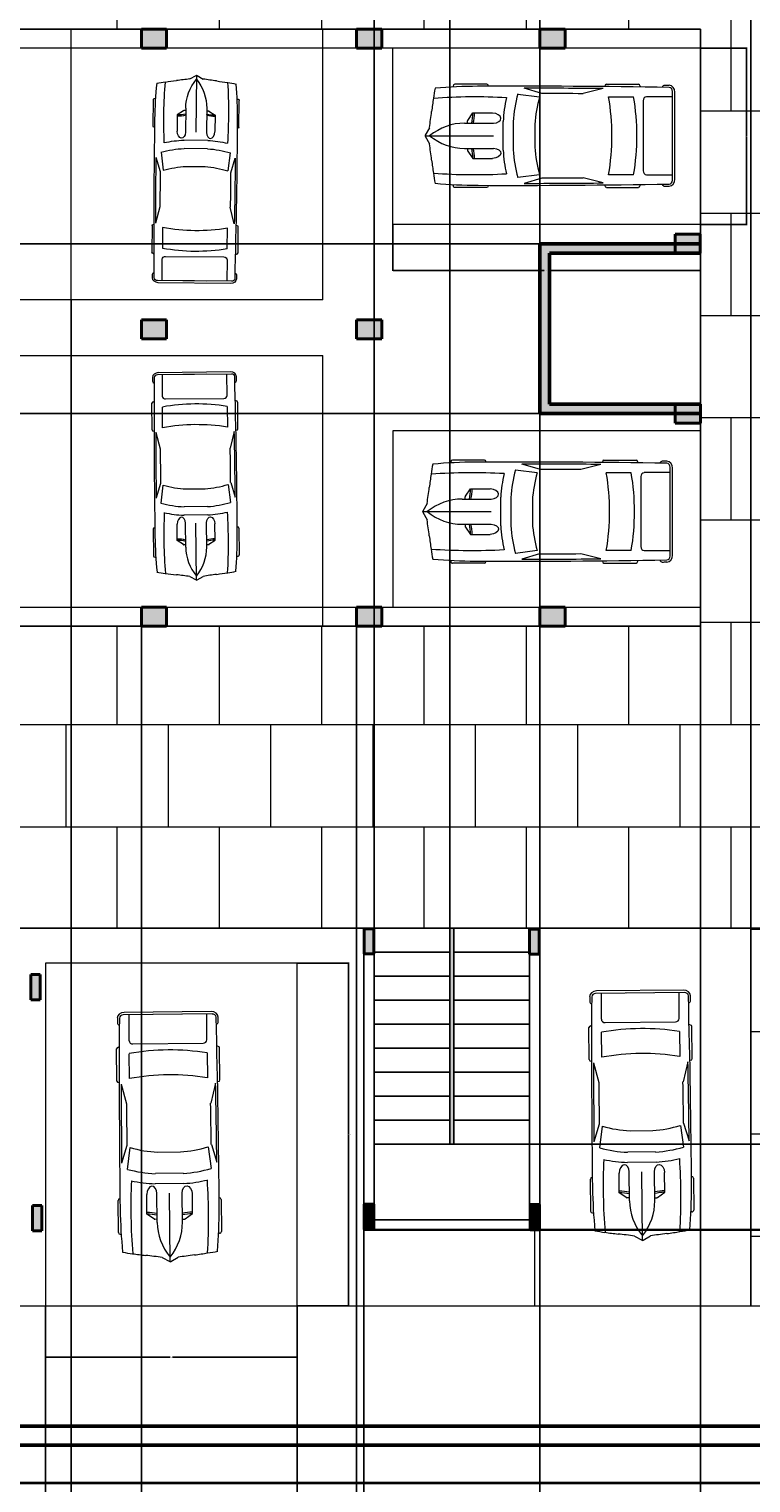
# Model space of a CAD drawing. Units: inches. Extents: x 154617 to 156384, y 250671 to 252576.
# Tile 4 of 6: x 155601 to 155945, y 251035 to 251728. Entities that reach past the tile are written whole.
import ezdxf

# ---------------------------------------------------------------- set-up
doc = ezdxf.new("R2010")
doc.units = ezdxf.units.IN
for name, color, linetype, lineweight in [('A-ANNO-DIMS', 2, 'Continuous', 18), ('A-COLS-PATT', 6, 'Continuous', 13), ('A-EQPM-VEHI', 9, 'Continuous', 13), ('A-FLOR-DRIV', 5, 'Continuous', 25), ('A-FLOR-PATT', 112, 'Continuous', 13), ('A-FLOR-PRKG', 4, 'Continuous', 18), ('A-FLOR-STRS', 7, 'Continuous', 25), ('A-FLOR-STRS-PATT', 20, 'Continuous', 13), ('A-WALL-PATT', 8, 'Continuous', 13), ('C-PROP', 5, 'Continuous', 35), ('pillars', 6, 'Continuous', 40), ('walls', 4, 'Continuous', 50)]:
    doc.layers.add(name, color=color, linetype=linetype, lineweight=lineweight)
doc.styles.get("Standard").update_dxf_attribs({"font": 'arial.ttf'})
doc.dimstyles.get("Standard").update_dxf_attribs({"dimtxt": 0.18, "dimasz": 0.18, "dimexe": 0.18, "dimexo": 0.0625, "dimgap": 0.09, "dimtad": 0, "dimtih": 1, "dimtoh": 1, "dimdec": 4, "dimzin": 0, "dimdsep": 46, "dimtxsty": 'Standard', "dimcen": 0.09, "dimadec": 0, "dimazin": 0, "dimtfac": 1, "dimtdec": 4, "dimtofl": 0, "dimtmove": 0, "dimatfit": 3, "dimfxl": 1, "dimtolj": 1, "dimtzin": 0, "dimarcsym": 0})

# ---------------------------------------------------------------- blocks, each defined once
blk = doc.blocks.new('*U2')
for p, q in [((21.1, 37.4), (21.1, 36.8)), ((46.6, 38.9), (22.4, 38.9)), ((47.8, 37.4), (47.8, 37.4)), ((88, 31.9), (74.8, 35.9)), ((134.3, 35.6), (119.3, 31.8)), ((135.5, 37.1), (135.5, 37.4)), ((136.7, 38.9), (160.9, 38.9)), ((162.1, 37.4), (162.1, 36.8)), ((186.5, -33.5), (186.5, 33.5)), ((70, 31.5), (86.4, 29.4)), ((138.4, 29.4), (157.2, 29.4)), ((164.5, 26.4), (164.5, -26.4)), ((186.5, 29.4), (167, 29.4)), ((188.4, -32.8), (188.4, 32.8)), ((32.1, 9.5), (32.1, 11.2)), ((32.3, 11.6), (36.1, 17.2)), ((36.1, 17.2), (50.9, 17.2)), ((3.3, 6.1), (0.1, 0.4)), ((29.8, 9.5), (51.7, 9.5)), ((58.9, -10.8), (58.9, 10.8)), ((66.6, -10.5), (66.6, 10.5)), ((82.7, 8.5), (82.7, -8.5)), ((186.5, -10.5), (186.5, 10.5)), ((0, 0), (51.7, 0)), ((0.1, -0.4), (3.3, -6.1)), ((29.8, -9.5), (51.7, -9.5)), ((32.1, -9.5), (32.1, -11.2)), ((32.3, -11.6), (36.1, -17.2)), ((36.1, -17.2), (50.9, -17.2)), ((86.4, -29.4), (70, -31.5)), ((88, -31.9), (74.8, -35.9)), ((134.3, -35.6), (119.3, -31.8)), ((157.2, -29.4), (138.4, -29.4)), ((167, -29.4), (186.5, -29.4)), ((21.1, -37.4), (21.1, -36.8)), ((46.6, -38.9), (22.4, -38.9)), ((47.8, -37.4), (47.8, -37.4)), ((135.5, -37.1), (135.5, -37.4)), ((136.7, -38.9), (160.9, -38.9)), ((162.1, -37.4), (162.1, -36.8))]:
    blk.add_line(p, q)
for centre, major_axis, ratio, start_param, end_param in [((266, -27.5), (0, 313.3), 0.842304, 1.367076, 1.39176), ((41.2, -490.9), (0, 528.2), 0.842304, 0.00281, 0.075598), ((22.4, 37.4), (0, -1.48), 0.842304, 3.141593, 4.712389), ((64.5, -10555.6), (0, 10593), 0.842304, -0.013397, 0.002797), ((46.6, 37.4), (0, 1.48), 0.842304, -1.570796, 0), ((64.5, -10555.6), (0, -10591.5), 0.842304, 3.133765, 3.140441), ((136.7, 37.4), (0, -1.48), 0.842304, 3.141593, 4.712389), ((160.9, 37.4), (0, 1.48), 0.842304, -1.570796, 0), ((180.6, 35.8), (0, 2.22), 0.842304, -0.013017, 1.249894), ((64.5, -10556.4), (0, 10595.3), 0.842304, -0.013397, -0.013017), ((184, 32.8), (0, -5.25), 0.842304, 1.570796, 3.128196), ((184, 33.5), (0, -2.96), 0.842304, 1.570796, 3.128196), ((259.2, -27.5), (0, -305.3), 0.842304, 4.528606, 4.561838), ((37.5, -594), (0, -623.3), 0.842304, 3.096046, 3.200911), ((134.4, 5.4), (0, -89.8), 0.842304, 4.449482, 4.652344), ((135.3, 5.4), (0, 81.8), 0.842304, 1.245306, 1.50788), ((149.6, 2.8), (0, -79.6), 0.842304, 4.372215, 4.640744), ((95.8, -3666.4), (0, -3698.2), 0.842304, 3.134049, 3.144098), ((17.1, 0), (0, 147), 0.842304, 4.511394, 4.913384), ((35.9, 0), (0, 147), 0.842304, 4.511394, 4.913384), ((167, 26.4), (0, 2.96), 0.842304, 0, 1.570796), ((-204.5, 52.4), (0, -251), 0.842304, 1.385369, 1.434372), ((32.7, 11.2), (0, 0.74), 0.842304, 0.879714, 1.570796), ((13, 17), (0, 27.4), 0.842304, 4.435146, 4.718221), ((14.2, 17), (0, 27.4), 0.842304, 4.435146, 4.718221), ((50.8, 13.3), (6.34, -0.36), 0.603834, -1.395552, 1.581315), ((0.6, 0), (0, -0.74), 0.842304, 4.131459, 5.293319), ((29.8, -46.7), (0, 56.2), 0.842304, 0, 0.590319), ((-204.5, -52.4), (0, 251), 0.842304, -1.434372, -1.385369), ((29.8, 46.7), (0, 56.2), 0.842304, 2.551274, 3.141593), ((13, -17), (0, -27.4), 0.842304, 1.564964, 1.848039), ((14.2, -17), (0, -27.4), 0.842304, 1.564964, 1.848039), ((134.4, -5.4), (0, -89.8), 0.842304, -1.510751, -1.307889), ((135.3, -5.4), (0, -81.8), 0.842304, -1.50788, -1.245306), ((149.6, -2.8), (0, -79.6), 0.842304, -1.499151, -1.230623), ((259.2, 27.5), (0, 305.3), 0.842304, 1.721348, 1.754579), ((32.7, -11.2), (0, -0.74), 0.842304, 4.712389, 5.403472), ((266, 27.5), (0, 313.3), 0.842304, 1.749832, 1.774517), ((37.5, 594), (0, -623.3), 0.842304, -0.059319, 0.045547), ((95.8, 3666.4), (0, -3698.2), 0.842304, -0.002505, 0.007544), ((167, -26.4), (0, -2.96), 0.842304, 4.712389, 6.283185), ((184, -32.8), (0, -5.25), 0.842304, 0.013397, 1.570796), ((41.2, 490.9), (0, -528.2), 0.842304, -0.075598, -0.00281), ((22.4, -37.4), (0, 1.48), 0.842304, 1.570796, 3.141593), ((64.5, 10555.6), (0, 10593), 0.842304, 3.138796, 3.15499), ((46.6, -37.4), (0, -1.48), 0.842304, 0, 1.570796), ((64.5, 10555.6), (0, -10591.5), 0.842304, 0.001152, 0.007828), ((136.7, -37.4), (0, -1.48), 0.842304, -1.570796, 0), ((160.9, -37.4), (0, 1.48), 0.842304, 3.141593, 4.712389), ((180.6, -35.8), (0, -2.22), 0.842304, -1.249894, 0.013017), ((64.5, 10556.4), (0, 10595.3), 0.842304, 3.15461, 3.15499), ((184, -33.5), (0, 2.96), 0.842304, 3.15499, 4.712389)]:
    blk.add_ellipse(centre, major_axis=major_axis, ratio=ratio, start_param=start_param, end_param=end_param)
at = {"extrusion": (0, 0, -1)}
blk.add_ellipse((50.8, -13.3), major_axis=(6.34, 0.36), ratio=0.603834, start_param=-1.395552, end_param=1.581315, dxfattribs=at)
blk = doc.blocks.new('COL-RECT-12x9')
h = blk.add_hatch(color=256)
h.dxf.hatch_style = 1
h.paths.add_polyline_path([(12.01, 0), (12.01, 9), (0, 9), (0, 0)])
for p, q in [((12.01, 9), (0, 9)), ((0, 9), (0, 0)), ((12.01, 0), (12.01, 9)), ((0, 0), (12.01, 0))]:
    blk.add_line(p, q)
blk = doc.blocks.new('COL-NARROW-4_5x12')
h = blk.add_hatch(color=256)
h.dxf.hatch_style = 1
h.paths.add_polyline_path([(4.5, 12.01), (0, 12.01), (0, 0), (4.5, 0)])
for p, q in [((4.5, 12.01), (0, 12.01)), ((0, 12.01), (0, 0)), ((4.5, 0), (4.5, 12.01)), ((0, 0), (4.5, 0))]:
    blk.add_line(p, q)
blk = doc.blocks.new('PARKING-BAY-U')
for p, q in [((120, 163.22), (0, 163.22)), ((0, 163.22), (0, 0)), ((120, 0), (120, 163.22))]:
    blk.add_line(p, q)
blk = doc.blocks.new('PARKING-BAY-L')
for p, q in [((0, 0), (0, 84)), ((146.69, 0), (0, 0))]:
    blk.add_line(p, q)
blk = doc.blocks.new('*D15')
at = {"layer": 'A-ANNO-DIMS', "color": 0, "lineweight": -2, "transparency": 16777216}
for p, q in [((155728.99, 251282.75), (155753.59, 251282.75)), ((155753.41, 251282.57), (155753.41, 251201.32)), ((155753.41, 251119.71), (155753.41, 251200.96)), ((155728.99, 251119.53), (155753.59, 251119.53))]:
    blk.add_line(p, q, dxfattribs=at)
at = {"layer": 'A-ANNO-DIMS', "color": 0, "transparency": 16777216}
for points in [[(155753.38, 251282.57), (155753.44, 251282.57), (155753.41, 251282.75)], [(155753.38, 251119.71), (155753.44, 251119.71), (155753.41, 251119.53)]]:
    blk.add_solid(points, dxfattribs=at)
at = {"layer": 'Defpoints', "color": 0, "transparency": 16777216}
for p in [(155728.93, 251282.75), (155753.41, 251282.75), (155728.93, 251119.53)]:
    blk.add_point(p, dxfattribs=at)
at = {"layer": 'A-ANNO-DIMS', "color": 0, "transparency": 16777216, "insert": (155753.41, 251201.14), "char_height": 0.18, "attachment_point": 5}
blk.add_mtext('\\A1;END BAY 163 TYP.', dxfattribs=at)
blk = doc.blocks.new('*D16')
at = {"layer": 'A-ANNO-DIMS', "color": 0, "lineweight": -2, "transparency": 16777216}
for p, q in [((155608.93, 251119.46), (155608.93, 251094.86)), ((155728.93, 251119.46), (155728.93, 251094.86)), ((155609.11, 251095.04), (155668.34, 251095.04)), ((155728.75, 251095.04), (155669.52, 251095.04))]:
    blk.add_line(p, q, dxfattribs=at)
at = {"layer": 'A-ANNO-DIMS', "color": 0, "transparency": 16777216}
for points in [[(155609.11, 251095.07), (155609.11, 251095.01), (155608.93, 251095.04)], [(155728.75, 251095.07), (155728.75, 251095.01), (155728.93, 251095.04)]]:
    blk.add_solid(points, dxfattribs=at)
at = {"layer": 'Defpoints', "color": 0, "transparency": 16777216}
for p in [(155608.93, 251119.53), (155728.93, 251119.53), (155728.93, 251095.04)]:
    blk.add_point(p, dxfattribs=at)
at = {"layer": 'A-ANNO-DIMS', "color": 0, "transparency": 16777216, "insert": (155668.93, 251095.04), "char_height": 0.18, "attachment_point": 5}
blk.add_mtext('\\A1;120 TYP.', dxfattribs=at)
blk = doc.blocks.new('*D17')
at = {"layer": 'A-ANNO-DIMS', "color": 0, "lineweight": -2, "transparency": 16777216}
for p, q in [((155774.41, 251634.96), (155774.41, 251612.84)), ((155921.1, 251634.96), (155921.1, 251612.84)), ((155774.59, 251613.02), (155846.54, 251613.02)), ((155920.92, 251613.02), (155848.96, 251613.02))]:
    blk.add_line(p, q, dxfattribs=at)
at = {"layer": 'A-ANNO-DIMS', "color": 0, "transparency": 16777216}
for points in [[(155774.59, 251613.05), (155774.59, 251612.99), (155774.41, 251613.02)], [(155920.92, 251613.05), (155920.92, 251612.99), (155921.1, 251613.02)]]:
    blk.add_solid(points, dxfattribs=at)
at = {"layer": 'Defpoints', "color": 0, "transparency": 16777216}
for p in [(155774.41, 251635.03), (155921.1, 251635.03), (155921.1, 251613.02)]:
    blk.add_point(p, dxfattribs=at)
at = {"layer": 'A-ANNO-DIMS', "color": 0, "transparency": 16777216, "insert": (155847.75, 251613.02), "char_height": 0.18, "attachment_point": 5}
blk.add_mtext('\\A1;SIDE BAY 147 TYP.', dxfattribs=at)
blk = doc.blocks.new('*D18')
at = {"layer": 'A-ANNO-DIMS', "color": 0, "lineweight": -2, "transparency": 16777216}
for p, q in [((155921.16, 251719.03), (155943.28, 251719.03)), ((155943.1, 251718.85), (155943.1, 251677.21)), ((155943.1, 251635.21), (155943.1, 251676.84)), ((155921.16, 251635.03), (155943.28, 251635.03))]:
    blk.add_line(p, q, dxfattribs=at)
at = {"layer": 'A-ANNO-DIMS', "color": 0, "transparency": 16777216}
for points in [[(155943.07, 251718.85), (155943.13, 251718.85), (155943.1, 251719.03)], [(155943.07, 251635.21), (155943.13, 251635.21), (155943.1, 251635.03)]]:
    blk.add_solid(points, dxfattribs=at)
at = {"layer": 'Defpoints', "color": 0, "transparency": 16777216}
for p in [(155921.1, 251719.03), (155943.1, 251719.03), (155921.1, 251635.03)]:
    blk.add_point(p, dxfattribs=at)
at = {"layer": 'A-ANNO-DIMS', "color": 0, "transparency": 16777216, "insert": (155943.1, 251677.03), "char_height": 0.18, "attachment_point": 5}
blk.add_mtext('\\A1;84 TYP.', dxfattribs=at)
blk = doc.blocks.new('*D37')
at = {"layer": 'A-ANNO-DIMS', "color": 0, "lineweight": -2, "transparency": 16777216}
for p, q in [((155475.98, 251443.46), (155475.98, 250671.2)), ((155654.61, 251443.46), (155654.61, 250671.2)), ((155476.16, 250671.38), (155564.84, 250671.38)), ((155654.43, 250671.38), (155565.75, 250671.38))]:
    blk.add_line(p, q, dxfattribs=at)
at = {"layer": 'A-ANNO-DIMS', "color": 0, "transparency": 16777216}
for points in [[(155476.16, 250671.41), (155476.16, 250671.35), (155475.98, 250671.38)], [(155654.43, 250671.41), (155654.43, 250671.35), (155654.61, 250671.38)]]:
    blk.add_solid(points, dxfattribs=at)
at = {"layer": 'Defpoints', "color": 0, "transparency": 16777216}
for p in [(155475.98, 251443.53), (155654.61, 251443.53), (155654.61, 250671.38)]:
    blk.add_point(p, dxfattribs=at)
at = {"layer": 'A-ANNO-DIMS', "color": 0, "transparency": 16777216, "insert": (155565.3, 250671.38), "char_height": 0.18, "attachment_point": 5}
blk.add_mtext('\\A1;178.63', dxfattribs=at)
blk = doc.blocks.new('*D38')
at = {"layer": 'A-ANNO-DIMS', "color": 0, "lineweight": -2, "transparency": 16777216}
for p, q in [((155654.61, 251443.46), (155654.61, 250671.2)), ((155757.2, 251443.46), (155757.2, 250671.2)), ((155654.79, 250671.38), (155705.45, 250671.38)), ((155757.02, 250671.38), (155706.36, 250671.38))]:
    blk.add_line(p, q, dxfattribs=at)
at = {"layer": 'A-ANNO-DIMS', "color": 0, "transparency": 16777216}
for points in [[(155654.79, 250671.41), (155654.79, 250671.35), (155654.61, 250671.38)], [(155757.02, 250671.41), (155757.02, 250671.35), (155757.2, 250671.38)]]:
    blk.add_solid(points, dxfattribs=at)
at = {"layer": 'Defpoints', "color": 0, "transparency": 16777216}
for p in [(155654.61, 251443.53), (155757.2, 251443.53), (155757.2, 250671.38)]:
    blk.add_point(p, dxfattribs=at)
at = {"layer": 'A-ANNO-DIMS', "color": 0, "transparency": 16777216, "insert": (155705.91, 250671.38), "char_height": 0.18, "attachment_point": 5}
blk.add_mtext('\\A1;102.59', dxfattribs=at)
blk = doc.blocks.new('*D39')
at = {"layer": 'A-ANNO-DIMS', "color": 0, "lineweight": -2, "transparency": 16777216}
for p, q in [((155757.2, 251443.46), (155757.2, 250671.2)), ((155844.6, 251443.46), (155844.6, 250671.2)), ((155757.38, 250671.38), (155800.58, 250671.38)), ((155844.42, 250671.38), (155801.22, 250671.38))]:
    blk.add_line(p, q, dxfattribs=at)
at = {"layer": 'A-ANNO-DIMS', "color": 0, "transparency": 16777216}
for points in [[(155757.38, 250671.41), (155757.38, 250671.35), (155757.2, 250671.38)], [(155844.42, 250671.41), (155844.42, 250671.35), (155844.6, 250671.38)]]:
    blk.add_solid(points, dxfattribs=at)
at = {"layer": 'Defpoints', "color": 0, "transparency": 16777216}
for p in [(155757.2, 251443.53), (155844.6, 251443.53), (155844.6, 250671.38)]:
    blk.add_point(p, dxfattribs=at)
at = {"layer": 'A-ANNO-DIMS', "color": 0, "transparency": 16777216, "insert": (155800.9, 250671.38), "char_height": 0.18, "attachment_point": 5}
blk.add_mtext('\\A1;87.4', dxfattribs=at)
blk = doc.blocks.new('*D52')
at = {"layer": 'A-ANNO-DIMS', "color": 0, "lineweight": -2, "transparency": 16777216}
for p, q in [((155760.6, 251155.46), (155760.6, 250671.2)), ((155844.6, 251155.46), (155844.6, 250671.2)), ((155760.78, 250671.38), (155802.38, 250671.38)), ((155844.42, 250671.38), (155802.82, 250671.38))]:
    blk.add_line(p, q, dxfattribs=at)
at = {"layer": 'A-ANNO-DIMS', "color": 0, "transparency": 16777216}
for points in [[(155760.78, 250671.41), (155760.78, 250671.35), (155760.6, 250671.38)], [(155844.42, 250671.41), (155844.42, 250671.35), (155844.6, 250671.38)]]:
    blk.add_solid(points, dxfattribs=at)
at = {"layer": 'Defpoints', "color": 0, "transparency": 16777216}
for p in [(155760.6, 251155.53), (155844.6, 251155.53), (155844.6, 250671.38)]:
    blk.add_point(p, dxfattribs=at)
at = {"layer": 'A-ANNO-DIMS', "color": 0, "transparency": 16777216, "insert": (155802.6, 250671.38), "char_height": 0.18, "attachment_point": 5}
blk.add_mtext('\\A1;84', dxfattribs=at)
blk = doc.blocks.new('*D53')
at = {"layer": 'A-ANNO-DIMS', "color": 0, "lineweight": -2, "transparency": 16777216}
for p, q in [((155844.66, 251299.53), (156383.38, 251299.53)), ((156383.2, 251299.35), (156383.2, 251227.71)), ((156383.2, 251155.71), (156383.2, 251227.35)), ((155844.66, 251155.53), (156383.38, 251155.53))]:
    blk.add_line(p, q, dxfattribs=at)
at = {"layer": 'A-ANNO-DIMS', "color": 0, "transparency": 16777216}
for points in [[(156383.17, 251299.35), (156383.23, 251299.35), (156383.2, 251299.53)], [(156383.17, 251155.71), (156383.23, 251155.71), (156383.2, 251155.53)]]:
    blk.add_solid(points, dxfattribs=at)
at = {"layer": 'Defpoints', "color": 0, "transparency": 16777216}
for p in [(155844.6, 251299.53), (156383.2, 251299.53), (155844.6, 251155.53)]:
    blk.add_point(p, dxfattribs=at)
at = {"layer": 'A-ANNO-DIMS', "color": 0, "transparency": 16777216, "insert": (156383.2, 251227.53), "char_height": 0.18, "attachment_point": 5}
blk.add_mtext('\\A1;144', dxfattribs=at)
blk = doc.blocks.new('*D54')
at = {"layer": 'A-ANNO-DIMS', "color": 0, "lineweight": -2, "transparency": 16777216}
for p, q in [((155844.6, 251544.74), (155844.6, 250671.2)), ((155921.1, 251544.74), (155921.1, 250671.2)), ((155844.78, 250671.38), (155882.52, 250671.38)), ((155920.92, 250671.38), (155883.17, 250671.38))]:
    blk.add_line(p, q, dxfattribs=at)
at = {"layer": 'A-ANNO-DIMS', "color": 0, "transparency": 16777216}
for points in [[(155844.78, 250671.41), (155844.78, 250671.35), (155844.6, 250671.38)], [(155920.92, 250671.41), (155920.92, 250671.35), (155921.1, 250671.38)]]:
    blk.add_solid(points, dxfattribs=at)
at = {"layer": 'Defpoints', "color": 0, "transparency": 16777216}
for p in [(155844.6, 251544.8), (155921.1, 251544.8), (155921.1, 250671.38)]:
    blk.add_point(p, dxfattribs=at)
at = {"layer": 'A-ANNO-DIMS', "color": 0, "transparency": 16777216, "insert": (155882.85, 250671.38), "char_height": 0.18, "attachment_point": 5}
blk.add_mtext('\\A1;76.5', dxfattribs=at)
blk = doc.blocks.new('*D55')
at = {"layer": 'A-ANNO-DIMS', "color": 0, "lineweight": -2, "transparency": 16777216}
for p, q in [((155844.53, 251625.8), (154616.73, 251625.8)), ((154616.91, 251625.62), (154616.91, 251585.48)), ((154616.91, 251544.98), (154616.91, 251585.12)), ((155844.53, 251544.8), (154616.73, 251544.8))]:
    blk.add_line(p, q, dxfattribs=at)
at = {"layer": 'A-ANNO-DIMS', "color": 0, "transparency": 16777216}
for points in [[(154616.88, 251625.62), (154616.94, 251625.62), (154616.91, 251625.8)], [(154616.88, 251544.98), (154616.94, 251544.98), (154616.91, 251544.8)]]:
    blk.add_solid(points, dxfattribs=at)
at = {"layer": 'Defpoints', "color": 0, "transparency": 16777216}
for p in [(154616.91, 251625.8), (155844.6, 251625.8), (155844.6, 251544.8)]:
    blk.add_point(p, dxfattribs=at)
at = {"layer": 'A-ANNO-DIMS', "color": 0, "transparency": 16777216, "insert": (154616.91, 251585.3), "char_height": 0.18, "attachment_point": 5}
blk.add_mtext('\\A1;81', dxfattribs=at)
blk = doc.blocks.new('*D57')
at = {"layer": 'A-ANNO-DIMS', "color": 0, "lineweight": -2, "transparency": 16777216}
for p, q in [((155480.24, 251119.46), (155480.24, 250671.2)), ((155608.93, 251119.46), (155608.93, 250671.2)), ((155480.42, 250671.38), (155544.13, 250671.38)), ((155608.75, 250671.38), (155545.04, 250671.38))]:
    blk.add_line(p, q, dxfattribs=at)
at = {"layer": 'A-ANNO-DIMS', "color": 0, "transparency": 16777216}
for points in [[(155480.42, 250671.41), (155480.42, 250671.35), (155480.24, 250671.38)], [(155608.75, 250671.41), (155608.75, 250671.35), (155608.93, 250671.38)]]:
    blk.add_solid(points, dxfattribs=at)
at = {"layer": 'Defpoints', "color": 0, "transparency": 16777216}
for p in [(155480.24, 251119.53), (155608.93, 251119.53), (155608.93, 250671.38)]:
    blk.add_point(p, dxfattribs=at)
at = {"layer": 'A-ANNO-DIMS', "color": 0, "transparency": 16777216, "insert": (155544.58, 250671.38), "char_height": 0.18, "attachment_point": 5}
blk.add_mtext('\\A1;128.68', dxfattribs=at)
blk = doc.blocks.new('*D58')
at = {"layer": 'A-ANNO-DIMS', "color": 0, "lineweight": -2, "transparency": 16777216}
for p, q in [((155844.6, 251299.59), (155844.6, 252576.18)), ((155844.78, 252576), (155894.46, 252576)), ((155944.92, 252576), (155895.23, 252576)), ((155945.1, 251299.59), (155945.1, 252576.18))]:
    blk.add_line(p, q, dxfattribs=at)
at = {"layer": 'A-ANNO-DIMS', "color": 0, "transparency": 16777216}
for points in [[(155844.78, 252576.03), (155844.78, 252575.97), (155844.6, 252576)], [(155944.92, 252576.03), (155944.92, 252575.97), (155945.1, 252576)]]:
    blk.add_solid(points, dxfattribs=at)
at = {"layer": 'Defpoints', "color": 0, "transparency": 16777216}
for p in [(155945.1, 252576), (155844.6, 251299.53), (155945.1, 251299.53)]:
    blk.add_point(p, dxfattribs=at)
at = {"layer": 'A-ANNO-DIMS', "color": 0, "transparency": 16777216, "insert": (155894.85, 252576), "char_height": 0.18, "attachment_point": 5}
blk.add_mtext('\\A1;100.5', dxfattribs=at)
blk = doc.blocks.new('*D61')
at = {"layer": 'A-ANNO-DIMS', "color": 0, "lineweight": -2, "transparency": 16777216}
for p, q in [((155501.1, 251598.96), (155501.1, 250671.2)), ((155621.1, 251598.96), (155621.1, 250671.2)), ((155501.28, 250671.38), (155560.82, 250671.38)), ((155620.92, 250671.38), (155561.38, 250671.38))]:
    blk.add_line(p, q, dxfattribs=at)
at = {"layer": 'A-ANNO-DIMS', "color": 0, "transparency": 16777216}
for points in [[(155501.28, 250671.41), (155501.28, 250671.35), (155501.1, 250671.38)], [(155620.92, 250671.41), (155620.92, 250671.35), (155621.1, 250671.38)]]:
    blk.add_solid(points, dxfattribs=at)
at = {"layer": 'Defpoints', "color": 0, "transparency": 16777216}
for p in [(155501.1, 251599.03), (155621.1, 251599.03), (155621.1, 250671.38)]:
    blk.add_point(p, dxfattribs=at)
at = {"layer": 'A-ANNO-DIMS', "color": 0, "transparency": 16777216, "insert": (155561.1, 250671.38), "char_height": 0.18, "attachment_point": 5}
blk.add_mtext('\\A1;120', dxfattribs=at)
blk = doc.blocks.new('*D68')
at = {"layer": 'A-ANNO-DIMS', "color": 0, "lineweight": -2, "transparency": 16777216}
for p, q in [((155760.6, 251155.46), (155760.6, 250671.2)), ((155728.93, 251119.46), (155728.93, 250671.2)), ((155729.11, 250671.38), (155744.37, 250671.38)), ((155760.42, 250671.38), (155745.16, 250671.38))]:
    blk.add_line(p, q, dxfattribs=at)
at = {"layer": 'A-ANNO-DIMS', "color": 0, "transparency": 16777216}
for points in [[(155729.11, 250671.41), (155729.11, 250671.35), (155728.93, 250671.38)], [(155760.42, 250671.41), (155760.42, 250671.35), (155760.6, 250671.38)]]:
    blk.add_solid(points, dxfattribs=at)
at = {"layer": 'Defpoints', "color": 0, "transparency": 16777216}
for p in [(155760.6, 251155.53), (155728.93, 251119.53), (155760.6, 250671.38)]:
    blk.add_point(p, dxfattribs=at)
at = {"layer": 'A-ANNO-DIMS', "color": 0, "transparency": 16777216, "insert": (155744.76, 250671.38), "char_height": 0.18, "attachment_point": 5}
blk.add_mtext('\\A1;31.67', dxfattribs=at)
blk = doc.blocks.new('*D69')
at = {"layer": 'A-ANNO-DIMS', "color": 0, "lineweight": -2, "transparency": 16777216}
for p, q in [((155765.66, 251196.53), (156383.38, 251196.53)), ((156383.2, 251196.35), (156383.2, 251176.37)), ((156383.2, 251156.03), (156383.2, 251176.01)), ((155765.41, 251155.85), (156383.38, 251155.85))]:
    blk.add_line(p, q, dxfattribs=at)
at = {"layer": 'A-ANNO-DIMS', "color": 0, "transparency": 16777216}
for points in [[(156383.17, 251196.35), (156383.23, 251196.35), (156383.2, 251196.53)], [(156383.17, 251156.03), (156383.23, 251156.03), (156383.2, 251155.85)]]:
    blk.add_solid(points, dxfattribs=at)
at = {"layer": 'Defpoints', "color": 0, "transparency": 16777216}
for p in [(155765.6, 251196.53), (156383.2, 251196.53), (155765.34, 251155.85)]:
    blk.add_point(p, dxfattribs=at)
at = {"layer": 'A-ANNO-DIMS', "color": 0, "transparency": 16777216, "insert": (156383.2, 251176.19), "char_height": 0.18, "attachment_point": 5}
blk.add_mtext('\\A1;40.67', dxfattribs=at)
blk = doc.blocks.new('*D70')
at = {"layer": 'A-ANNO-DIMS', "color": 0, "lineweight": -2, "transparency": 16777216}
for p, q in [((155765.6, 251299.59), (155765.6, 252576.18)), ((155765.78, 252576), (155783.38, 252576)), ((155801.42, 252576), (155783.82, 252576)), ((155801.6, 251299.59), (155801.6, 252576.18))]:
    blk.add_line(p, q, dxfattribs=at)
at = {"layer": 'A-ANNO-DIMS', "color": 0, "transparency": 16777216}
for points in [[(155765.78, 252576.03), (155765.78, 252575.97), (155765.6, 252576)], [(155801.42, 252576.03), (155801.42, 252575.97), (155801.6, 252576)]]:
    blk.add_solid(points, dxfattribs=at)
at = {"layer": 'Defpoints', "color": 0, "transparency": 16777216}
for p in [(155801.6, 252576), (155765.6, 251299.53), (155801.6, 251299.53)]:
    blk.add_point(p, dxfattribs=at)
at = {"layer": 'A-ANNO-DIMS', "color": 0, "transparency": 16777216, "insert": (155783.6, 252576), "char_height": 0.18, "attachment_point": 5}
blk.add_mtext('\\A1;36', dxfattribs=at)

msp = doc.modelspace()

# ---------------------------------------------------------------- hatches: boundary and pattern name
at = {"layer": 'A-COLS-PATT'}
h = msp.add_hatch(color=256, dxfattribs=at)
h.dxf.hatch_style = 1
h.paths.add_polyline_path([(155921.015, 251630.322), (155909.002, 251630.322), (155909.002, 251625.802), (155921.015, 251625.802)])
h = msp.add_hatch(color=256, dxfattribs=at)
h.dxf.hatch_style = 1
h.paths.add_polyline_path([(155921.07, 251544.802), (155909.057, 251544.802), (155909.057, 251540.302), (155921.07, 251540.302)])
h = msp.add_hatch(color=256, dxfattribs=at)
h.dxf.hatch_style = 1
h.paths.add_polyline_path([(155765.343, 251167.865), (155760.843, 251167.865), (155760.843, 251160.526), (155765.343, 251160.526)])
h = msp.add_hatch(color=256, dxfattribs=at)
h.dxf.hatch_style = 1
h.paths.add_polyline_path([(155844.407, 251167.728), (155839.907, 251167.728), (155839.907, 251160.526), (155844.407, 251160.526)])
h = msp.add_hatch(color=256, dxfattribs=at)
h.dxf.hatch_style = 1
h.paths.add_polyline_path([(155765.343, 251160.526), (155760.843, 251160.526), (155760.843, 251155.853), (155765.343, 251155.853)])
h = msp.add_hatch(color=256, dxfattribs=at)
h.dxf.hatch_style = 1
h.paths.add_polyline_path([(155844.407, 251160.526), (155839.907, 251160.526), (155839.907, 251155.715), (155844.407, 251155.715)])
at = {"layer": 'A-FLOR-PATT'}
h = msp.add_hatch(dxfattribs=at)
h.set_pattern_fill('AR-B88', color=256, scale=0.24)
h.set_pattern_definition([(0, (0, -2.5), (0, 48.768), []), (90, (0, -2.5), (-24.384, 48.768), [48.768, -48.768])])
h.paths.add_polyline_path([(155324.842, 251443.526), (155324.842, 251299.526), (155945.097, 251299.526), (155945.097, 251119.526), (156089.097, 251119.526), (156089.097, 252132.026), (155921.097, 252132.026), (155921.097, 251872.026), (155324.842, 251872.026), (155324.842, 251728.026), (155921.097, 251728.026), (155921.097, 251443.526)])
at = {"layer": 'A-FLOR-STRS-PATT'}
h = msp.add_hatch(color=256, dxfattribs=at)
h.dxf.hatch_style = 1
h.paths.add_polyline_path([(155803.597, 251299.526), (155801.597, 251299.526), (155801.597, 251196.526), (155803.597, 251196.526)])
at = {"layer": 'A-WALL-PATT'}
h = msp.add_hatch(color=256, dxfattribs=at)
h.dxf.hatch_style = 1
h.paths.add_polyline_path([(155921.097, 251549.302), (155849.097, 251549.302), (155849.097, 251621.302), (155921.097, 251621.302), (155921.097, 251625.802), (155844.597, 251625.802), (155844.597, 251544.802), (155921.097, 251544.802)])

# ---------------------------------------------------------------- linework, layer by layer
at = {"layer": 'A-FLOR-DRIV'}
for p, q in [((155921.097, 251728.026), (155324.842, 251728.026)), ((155921.097, 251443.526), (155921.097, 251728.026)), ((155324.842, 251443.526), (155921.097, 251443.526)), ((155324.842, 251299.526), (155945.097, 251299.526)), ((155945.097, 251119.526), (155945.097, 251299.526))]:
    msp.add_line(p, q, dxfattribs=at)
at = {"layer": 'A-FLOR-PRKG'}
for p, q in [((155621.097, 251599.026), (155621.097, 251728.026)), ((155741.097, 251599.026), (155741.097, 251728.026)), ((155921.097, 251719.026), (155324.842, 251719.026)), ((155741.097, 251599.026), (155324.842, 251599.026)), ((155324.842, 251572.526), (155741.097, 251572.526)), ((155621.097, 251443.526), (155621.097, 251572.526)), ((155741.097, 251443.526), (155741.097, 251572.526)), ((155324.842, 251452.526), (155921.097, 251452.526)), ((155841.905, 251155.526), (155841.905, 251119.526)), ((155262.097, 251119.526), (156089.097, 251119.526))]:
    msp.add_line(p, q, dxfattribs=at)
at = {"layer": 'A-FLOR-STRS'}
for p, q in [((155760.597, 251155.526), (155760.597, 251299.526)), ((155844.597, 251299.526), (155760.597, 251299.526)), ((155765.597, 251155.526), (155765.597, 251299.526)), ((155801.597, 251196.526), (155801.597, 251299.526)), ((155803.597, 251299.526), (155803.597, 251196.526)), ((155839.597, 251299.526), (155839.597, 251155.526)), ((155844.597, 251299.526), (155844.597, 251155.526)), ((155801.597, 251288.082), (155765.597, 251288.082)), ((155839.597, 251288.082), (155803.597, 251288.082)), ((155801.597, 251276.638), (155765.597, 251276.638)), ((155839.597, 251276.638), (155803.597, 251276.638)), ((155801.597, 251265.193), (155765.597, 251265.193)), ((155839.597, 251265.193), (155803.597, 251265.193)), ((155801.597, 251253.749), (155765.597, 251253.749)), ((155839.597, 251253.749), (155803.597, 251253.749)), ((155801.597, 251242.304), (155765.597, 251242.304)), ((155839.597, 251242.304), (155803.597, 251242.304)), ((155801.597, 251230.86), (155765.597, 251230.86)), ((155839.597, 251230.86), (155803.597, 251230.86)), ((155801.597, 251219.415), (155765.597, 251219.415)), ((155839.597, 251219.415), (155803.597, 251219.415)), ((155801.597, 251207.971), (155765.597, 251207.971)), ((155839.597, 251207.971), (155803.597, 251207.971)), ((155839.597, 251196.526), (155765.597, 251196.526)), ((155844.597, 251160.526), (155760.597, 251160.526)), ((155844.597, 251155.526), (155760.597, 251155.526))]:
    msp.add_line(p, q, dxfattribs=at)
at = {"layer": 'C-PROP'}
msp.add_line((155235.097, 251035.026), (156296.097, 251035.026), dxfattribs=at)
at = {"layer": 'pillars'}
for p, q in [((155921.015, 251630.322), (155909.002, 251630.322)), ((155909.002, 251630.322), (155909.002, 251621.322)), ((155921.015, 251621.322), (155921.015, 251630.322)), ((155909.002, 251621.322), (155921.015, 251621.322)), ((155921.07, 251549.302), (155909.057, 251549.302)), ((155909.057, 251549.302), (155909.057, 251540.302)), ((155921.07, 251540.302), (155921.07, 251549.302)), ((155909.057, 251540.302), (155921.07, 251540.302)), ((155765.343, 251167.865), (155760.843, 251167.865)), ((155760.843, 251167.865), (155760.843, 251155.853)), ((155765.343, 251155.853), (155765.343, 251167.865)), ((155844.407, 251167.728), (155839.907, 251167.728)), ((155839.907, 251167.728), (155839.907, 251155.715)), ((155844.407, 251155.715), (155844.407, 251167.728)), ((155760.843, 251155.853), (155765.343, 251155.853)), ((155839.907, 251155.715), (155844.407, 251155.715))]:
    msp.add_line(p, q, dxfattribs=at)
at = {"layer": 'walls'}
for p, q in [((155844.597, 251544.802), (155844.597, 251625.802)), ((155844.597, 251625.802), (155921.097, 251625.802)), ((155849.097, 251621.302), (155921.097, 251621.302)), ((155849.097, 251549.302), (155849.097, 251621.302)), ((155921.097, 251549.302), (155849.097, 251549.302)), ((155921.097, 251544.802), (155844.597, 251544.802)), ((155262.097, 251062.026), (156269.097, 251062.026)), ((155253.097, 251053.026), (156278.097, 251053.026))]:
    msp.add_line(p, q, dxfattribs=at)

# ---------------------------------------------------------------- block references
at = {"layer": 'A-EQPM-VEHI'}
for p, xscale, yscale, zscale, rotation in [((155680.917, 251706.094), -0.5257159977764584, 0.5257159977764586, 0.5257159977764586, 89.41840527650862), ((155680.917, 251465.459), 0.5257159977764586, 0.5257159977764586, 0.5257159977764586, 90.58159472349136), ((155893.473, 251150.654), 0.632208294406123, 0.632208294406123, 0.632208294406123, 90.58159472349136), ((155668.354, 251140.465), 0.632208294406123, 0.632208294406123, 0.632208294406123, 90.58159472349136)]:
    msp.add_blockref('*U2', p, dxfattribs=dict(at, xscale=xscale, yscale=yscale, zscale=zscale, rotation=rotation))
at = {"layer": 'A-EQPM-VEHI', "xscale": 0.632208294406123, "yscale": 0.632208294406123, "zscale": 0.632208294406123}
for p in [(155789.808, 251677.265), (155788.682, 251498.08)]:
    msp.add_blockref('*U2', p, dxfattribs=at)
at = {"layer": 'A-FLOR-PRKG'}
for name, p in [('PARKING-BAY-L', (155774.408, 251635.026)), ('PARKING-BAY-U', (155608.926, 251119.526))]:
    msp.add_blockref(name, p, dxfattribs=at)
at = {"layer": 'A-FLOR-PRKG', "extrusion": (0, 0, -1), "zscale": -1, "rotation": 180}
msp.add_blockref('PARKING-BAY-L', (-155774.408, 251536.527), dxfattribs=at)
at = {"layer": 'pillars'}
for name, p in [('COL-RECT-12x9', (155654.613, 251719.027)), ('COL-RECT-12x9', (155757.202, 251719.027)), ('COL-RECT-12x9', (155844.597, 251719.027)), ('COL-RECT-12x9', (155654.613, 251580.536)), ('COL-RECT-12x9', (155757.202, 251580.536)), ('COL-RECT-12x9', (155654.613, 251443.527)), ('COL-RECT-12x9', (155757.202, 251443.527)), ('COL-RECT-12x9', (155844.597, 251443.527)), ('COL-NARROW-4_5x12', (155839.641, 251287.076))]:
    msp.add_blockref(name, p, dxfattribs=at)
at = {"layer": 'pillars', "rotation": 180}
for p in [(155765.332, 251299.234), (155606.44, 251277.342), (155607.218, 251167.287)]:
    msp.add_blockref('COL-NARROW-4_5x12', p, dxfattribs=at)

# ---------------------------------------------------------------- dimensions: what is measured, and where the dimension line sits
at = {"layer": 'A-ANNO-DIMS'}
for base, p1, p2, override, picture, middle in [((155801.597, 252575.997), (155765.597, 251299.526), (155801.597, 251299.526), {"dimdec": 0, "dimlfac": 1, "dimrnd": 0, "dimzin": 0, "dimdsep": 46, "dimlunit": 2}, '*D70', (155783.597, 252575.997)), ((155945.097, 252575.997), (155844.597, 251299.526), (155945.097, 251299.526), {"dimdec": 1, "dimlfac": 1, "dimrnd": 0, "dimzin": 0, "dimdsep": 46, "dimlunit": 2}, '*D58', (155894.847, 252575.997)), ((155621.097, 250671.379), (155501.097, 251599.026), (155621.097, 251599.026), {"dimdec": 0, "dimlfac": 1, "dimrnd": 0, "dimzin": 0, "dimdsep": 46, "dimlunit": 2}, '*D61', (155561.097, 250671.379)), ((155921.097, 250671.379), (155844.597, 251544.802), (155921.097, 251544.802), {"dimdec": 1, "dimlfac": 1, "dimrnd": 0, "dimzin": 0, "dimdsep": 46, "dimlunit": 2}, '*D54', (155882.847, 250671.379)), ((155654.613, 250671.379), (155475.98, 251443.526), (155654.613, 251443.526), {"dimdec": 2, "dimlfac": 1, "dimrnd": 0, "dimzin": 0, "dimdsep": 46, "dimlunit": 2}, '*D37', (155565.297, 250671.379)), ((155757.203, 250671.379), (155654.613, 251443.526), (155757.203, 251443.526), {"dimdec": 2, "dimlfac": 1, "dimrnd": 0, "dimzin": 0, "dimdsep": 46, "dimlunit": 2}, '*D38', (155705.908, 250671.379)), ((155844.597, 250671.379), (155757.203, 251443.526), (155844.597, 251443.526), {"dimdec": 1, "dimlfac": 1, "dimrnd": 0, "dimzin": 0, "dimdsep": 46, "dimlunit": 2}, '*D39', (155800.9, 250671.379)), ((155760.597, 250671.379), (155728.926, 251119.526), (155760.597, 251155.526), {"dimdec": 2, "dimlfac": 1, "dimrnd": 0, "dimzin": 0, "dimdsep": 46, "dimlunit": 2}, '*D68', (155744.761, 250671.379)), ((155844.597, 250671.379), (155760.597, 251155.526), (155844.597, 251155.526), {"dimdec": 0, "dimlfac": 1, "dimrnd": 0, "dimzin": 0, "dimdsep": 46, "dimlunit": 2}, '*D52', (155802.597, 250671.379)), ((155608.926, 250671.379), (155480.244, 251119.526), (155608.926, 251119.526), {"dimdec": 2, "dimlfac": 1, "dimrnd": 0, "dimzin": 0, "dimdsep": 46, "dimlunit": 2}, '*D57', (155544.585, 250671.379))]:
    dim = msp.add_linear_dim(base=base, p1=p1, p2=p2, dimstyle='Standard', override=override, dxfattribs=at)
    dim.commit()
    dim.dimension.update_dxf_attribs({"geometry": picture, "text_midpoint": middle})
for base, p1, p2, text, picture, middle in [((155943.101, 251719.026), (155921.097, 251635.026), (155921.097, 251719.026), '<> TYP.', '*D18', (155943.101, 251677.026)), ((155753.409, 251282.749), (155728.926, 251119.526), (155728.926, 251282.749), 'END BAY <> TYP.', '*D15', (155753.409, 251201.138))]:
    dim = msp.add_linear_dim(base=base, p1=p1, p2=p2, angle=90, text=text, dimstyle='Standard', override={"dimdec": 0, "dimlfac": 1, "dimrnd": 0, "dimzin": 0, "dimdsep": 46, "dimlunit": 2}, dxfattribs=at)
    dim.commit()
    dim.dimension.update_dxf_attribs({"geometry": picture, "text_midpoint": middle})
for base, p1, p2, text, picture, middle in [((155921.097, 251613.023), (155774.408, 251635.026), (155921.097, 251635.026), 'SIDE BAY <> TYP.', '*D17', (155847.752, 251613.023)), ((155728.926, 251095.043), (155608.926, 251119.526), (155728.926, 251119.526), '<> TYP.', '*D16', (155668.926, 251095.043))]:
    dim = msp.add_linear_dim(base=base, p1=p1, p2=p2, text=text, dimstyle='Standard', override={"dimdec": 0, "dimlfac": 1, "dimrnd": 0, "dimzin": 0, "dimdsep": 46, "dimlunit": 2}, dxfattribs=at)
    dim.commit()
    dim.dimension.update_dxf_attribs({"geometry": picture, "text_midpoint": middle})
for base, p1, p2, override, picture, middle in [((154616.915, 251625.802), (155844.597, 251544.802), (155844.597, 251625.802), {"dimdec": 0, "dimlfac": 1, "dimrnd": 0, "dimzin": 0, "dimdsep": 46, "dimlunit": 2}, '*D55', (154616.915, 251585.302)), ((156383.197, 251299.526), (155844.597, 251155.526), (155844.597, 251299.526), {"dimdec": 0, "dimlfac": 1, "dimrnd": 0, "dimzin": 0, "dimdsep": 46, "dimlunit": 2}, '*D53', (156383.197, 251227.526)), ((156383.197, 251196.526), (155765.343, 251155.853), (155765.597, 251196.526), {"dimdec": 2, "dimlfac": 1, "dimrnd": 0, "dimzin": 0, "dimdsep": 46, "dimlunit": 2}, '*D69', (156383.197, 251176.189))]:
    dim = msp.add_linear_dim(base=base, p1=p1, p2=p2, angle=90, dimstyle='Standard', override=override, dxfattribs=at)
    dim.commit()
    dim.dimension.update_dxf_attribs({"geometry": picture, "text_midpoint": middle})

doc.saveas('drawing.dxf')
